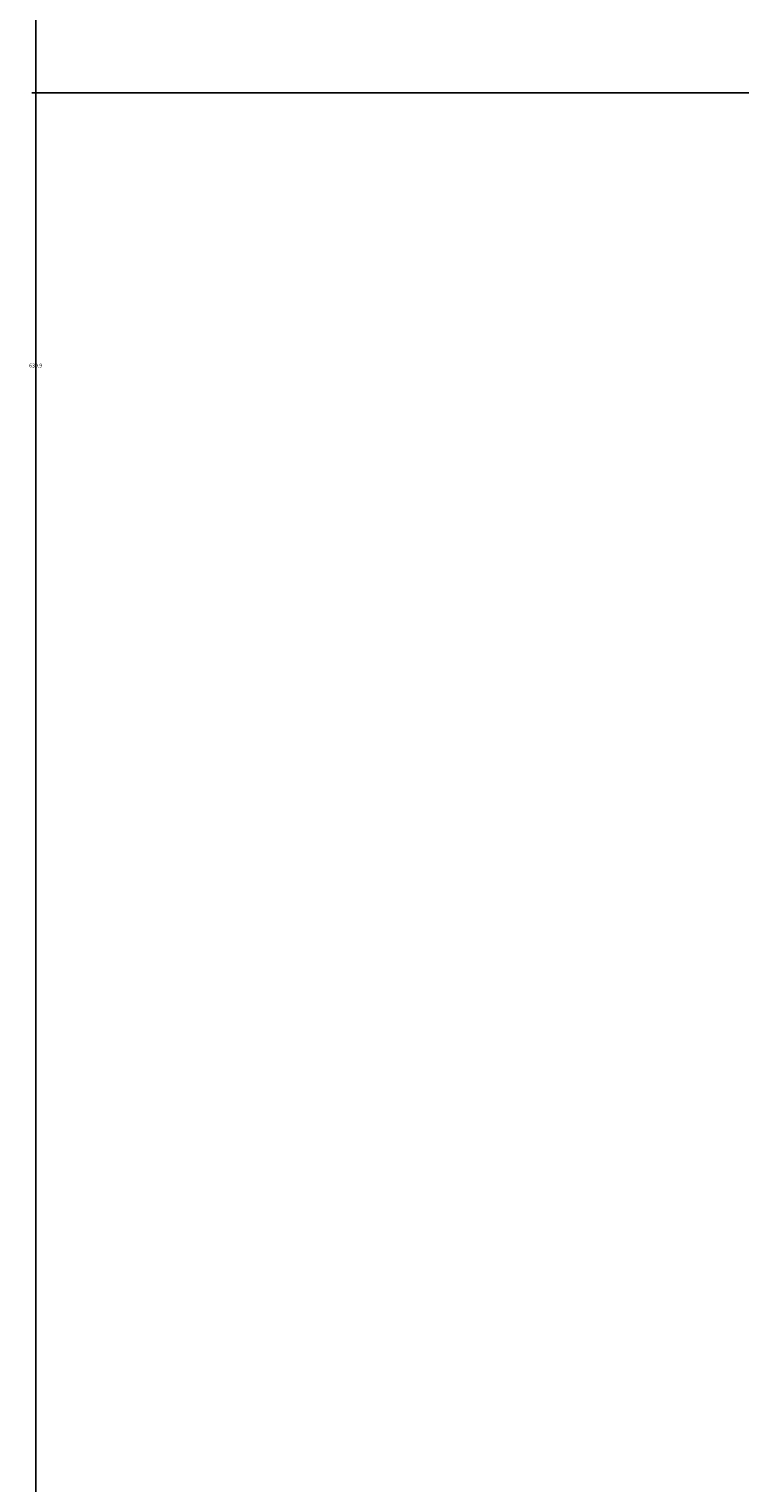
# Model space of a CAD drawing. Units: inches. Extents: x 4159 to 4826, y 299 to 1026.
# Tile 12 of 37: x 4159 to 4192, y 596 to 663. Entities that reach past the tile are written whole.
import ezdxf

# ---------------------------------------------------------------- set-up
doc = ezdxf.new("R2010")
doc.units = ezdxf.units.IN
doc.layers.add('A-ANNO-DIMS', color=2, linetype='Continuous', lineweight=18)
doc.styles.get("Standard").update_dxf_attribs({"font": 'arial.ttf'})
doc.dimstyles.get("Standard").update_dxf_attribs({"dimtxt": 0.18, "dimasz": 0.18, "dimexe": 0.18, "dimexo": 0.0625, "dimgap": 0.09, "dimtad": 0, "dimtih": 1, "dimtoh": 1, "dimdec": 4, "dimzin": 0, "dimdsep": 46, "dimtxsty": 'Standard', "dimcen": 0.09, "dimadec": 0, "dimazin": 0, "dimtfac": 1, "dimtdec": 4, "dimtofl": 0, "dimtmove": 0, "dimatfit": 3, "dimfxl": 1, "dimtolj": 1, "dimtzin": 0, "dimarcsym": 0})

# ---------------------------------------------------------------- blocks, each defined once
blk = doc.blocks.new('*D44')
at = {"layer": 'A-ANNO-DIMS', "color": 0, "lineweight": -2, "transparency": 16777216}
for p, q in [((4287.263, 963.093), (4158.88, 963.093)), ((4159.06, 962.913), (4159.06, 647.826)), ((4159.06, 332.375), (4159.06, 647.462)), ((4447.248, 332.195), (4158.88, 332.195))]:
    blk.add_line(p, q, dxfattribs=at)
at = {"layer": 'A-ANNO-DIMS', "color": 0, "transparency": 16777216}
for points in [[(4159.03, 962.913), (4159.09, 962.913), (4159.06, 963.093)], [(4159.03, 332.375), (4159.09, 332.375), (4159.06, 332.195)]]:
    blk.add_solid(points, dxfattribs=at)
at = {"layer": 'Defpoints', "color": 0, "transparency": 16777216}
for p in [(4287.326, 963.093), (4159.06, 332.195), (4447.31, 332.195)]:
    blk.add_point(p, dxfattribs=at)
at = {"layer": 'A-ANNO-DIMS', "color": 0, "transparency": 16777216, "insert": (4159.06, 647.644), "char_height": 0.18, "attachment_point": 5}
blk.add_mtext('\\A1;630.9', dxfattribs=at)
blk = doc.blocks.new('*D51')
at = {"layer": 'A-ANNO-DIMS', "color": 0, "lineweight": -2, "transparency": 16777216}
for p, q in [((4201.248, 660.254), (4158.88, 660.254)), ((4159.06, 660.074), (4159.06, 526.436)), ((4159.06, 392.434), (4159.06, 526.072)), ((4192.248, 392.254), (4158.88, 392.254))]:
    blk.add_line(p, q, dxfattribs=at)
at = {"layer": 'A-ANNO-DIMS', "color": 0, "transparency": 16777216}
for points in [[(4159.03, 660.074), (4159.09, 660.074), (4159.06, 660.254)], [(4159.03, 392.434), (4159.09, 392.434), (4159.06, 392.254)]]:
    blk.add_solid(points, dxfattribs=at)
at = {"layer": 'Defpoints', "color": 0, "transparency": 16777216}
for p in [(4159.06, 660.254), (4201.31, 660.254), (4192.31, 392.254)]:
    blk.add_point(p, dxfattribs=at)
at = {"layer": 'A-ANNO-DIMS', "color": 0, "transparency": 16777216, "insert": (4159.06, 526.254), "char_height": 0.18, "attachment_point": 5}
blk.add_mtext('\\A1;268', dxfattribs=at)

msp = doc.modelspace()

# ---------------------------------------------------------------- dimensions: what is measured, and where the dimension line sits
at = {"layer": 'A-ANNO-DIMS'}
for base, p1, p2, override, picture, middle in [((4159.06, 332.195), (4287.326, 963.093), (4447.31, 332.195), {"dimdec": 1, "dimlfac": 1, "dimrnd": 0, "dimzin": 0, "dimdsep": 46, "dimlunit": 2}, '*D44', (4159.06, 647.644)), ((4159.06, 660.254), (4192.31, 392.254), (4201.31, 660.254), {"dimdec": 0, "dimlfac": 1, "dimrnd": 0, "dimzin": 0, "dimdsep": 46, "dimlunit": 2}, '*D51', (4159.06, 526.254))]:
    dim = msp.add_linear_dim(base=base, p1=p1, p2=p2, angle=90, dimstyle='Standard', override=override, dxfattribs=at)
    dim.commit()
    dim.dimension.update_dxf_attribs({"geometry": picture, "text_midpoint": middle})

doc.saveas('drawing.dxf')
